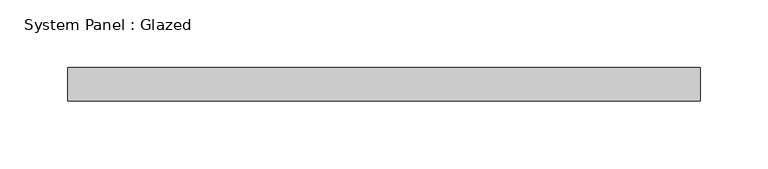
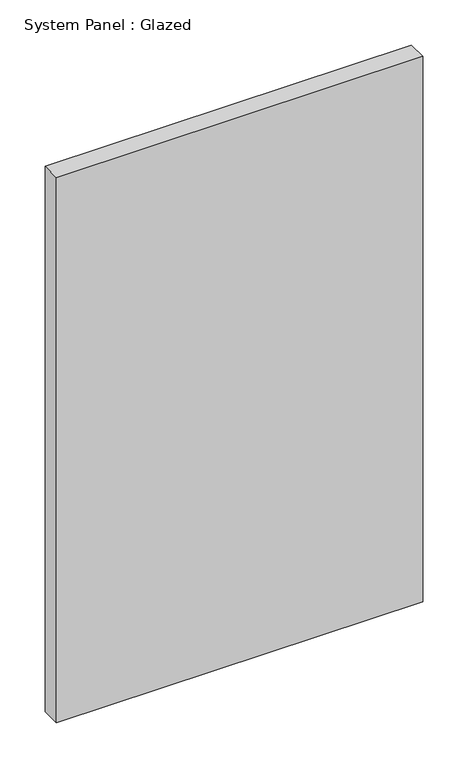
"""IFC4 building model written with IfcOpenShell, lengths in millimetres: plate geometry, System Panel : Glazed."""

from ifc_helpers import new_model, si_unit, origin, origin_with_axes, place, context, project, spatial, polyline, outline, extrude, source, transform, mapped, element, save


def system_panel_glazed_77a7bb99(model_context):
    return source(origin(), model_context, "Body", "SweptSolid", [
        extrude(outline(polyline([(234.0238623, 24.5), (-234.0238623, 24.5), (-234.0238623, 49.5), (234.0238623, 49.5), (234.0238623, 24.5)])), origin_with_axes(), (0.0, 0.0, 1.0), 736.6),
    ])


if __name__ == "__main__":
    model = new_model("IFC4")
    model_context = context("Model", 3, world=origin())
    ifc_project = project(units=[si_unit("LENGTHUNIT", "METRE", prefix="MILLI")], contexts=[model_context])
    site = spatial("IfcSite", under=ifc_project)
    building = spatial("IfcBuilding", under=site)
    placement = place(None, origin())
    system_panel_glazed_shape = system_panel_glazed_77a7bb99(model_context)
    element("IfcPlate", 1, ObjectType="System Panel : Glazed", at=placement, inside=building, context=model_context, shape_type="MappedRepresentation", body=[
        mapped(system_panel_glazed_shape, transform((0.0, 0.0, 0.0), x_axis=(1.0, 0.0, 0.0), y_axis=(0.0, 1.0, 0.0), z_axis=(0.0, 0.0, 1.0))),
    ])
    save(model, "model.ifc")

# Revit data of these elements
# Type "System Panel : Glazed"
#   Keynote = "H11"
#   Construction Type Id = "GSP4R"
#   Analytic Construction = "1/8 in Pilkington single glazing"
#   Visual Light Transmittance = 0.9
#   Solar Heat Gain Coefficient = 0.86
#   Heat Transfer Coefficient (U) = 6.7069 W/(m²·K)
#   Define Thermal Properties by = 1
# Element 1 (IfcPlate, "System Panel : Glazed")
#   Materials on its faces: "Glass"
# Materials
#   "Glass": class "Glass", colour RGB 0 128 192, transparency 0.9, Description = "Soda Lime Glass", Cost = 0
